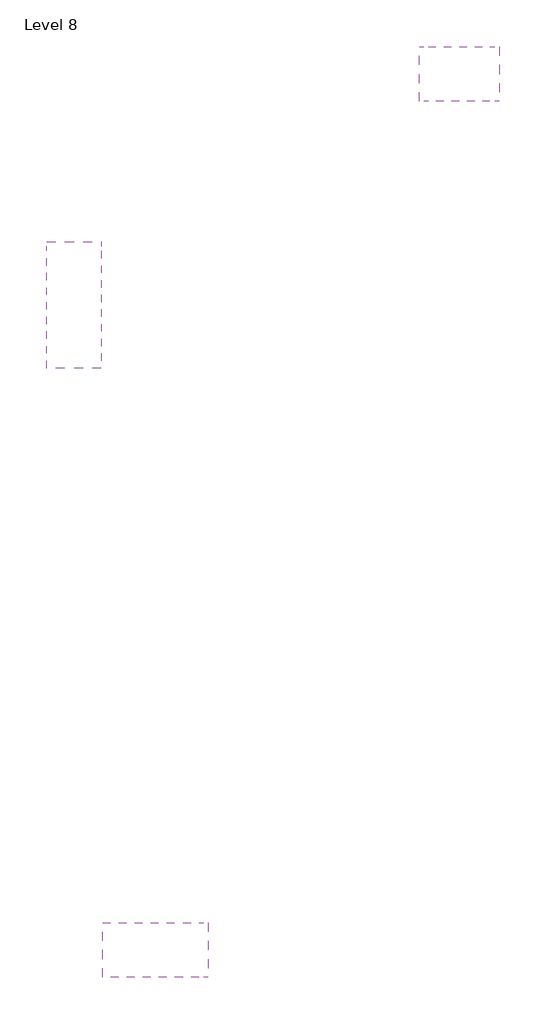
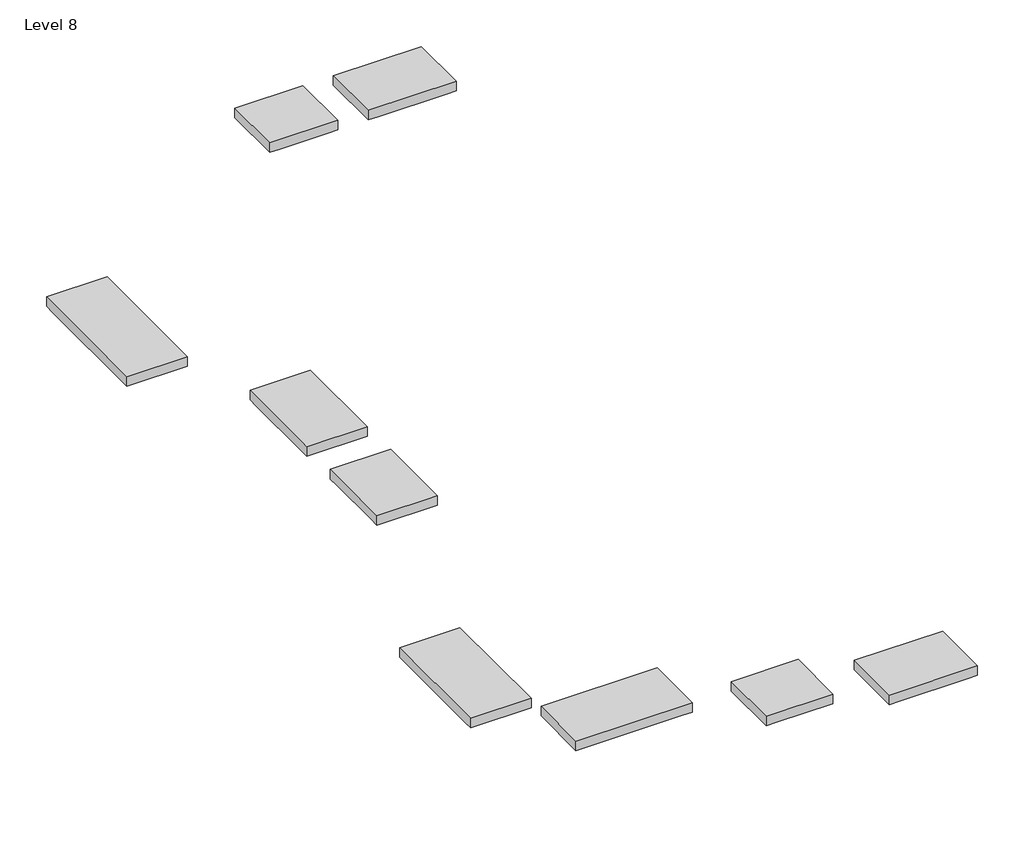
# One storey: 3 proxies.
"""IFC4 building model written with IfcOpenShell, lengths in millimetres."""

from ifc_helpers import new_model, si_unit, origin, place, context, project, spatial, transform, mapped, element, save
from components import generic_models_10_generic_models_10_998b1f2c, generic_models_11_generic_models_11_73ad1d2d, generic_models_12_generic_models_12_6034f315

model = new_model("IFC4")

# Units and contexts
model_context = context("Model", 3, world=origin())
ifc_project = project(units=[si_unit("LENGTHUNIT", "METRE", prefix="MILLI")], contexts=[model_context])

# Site, building, storey
site = spatial("IfcSite", under=ifc_project)
building = spatial("IfcBuilding", under=site)
storey = spatial("IfcBuildingStorey", under=building, Name="Level 8", Elevation=3962.4)

# Proxies
placement = place(None, origin())
generic_models_10_generic_models_10_shape = generic_models_10_generic_models_10_998b1f2c(model_context)
element("IfcBuildingElementProxy", 1, Name="Generic Models 10 : Generic Models 10", ObjectType="Generic Models 10 : Generic Models 10", at=placement, inside=storey, context=model_context, shape_type="MappedRepresentation", body=[
    mapped(generic_models_10_generic_models_10_shape, transform((0.0, 0.0, 0.0), x_axis=(1.0, 0.0, 0.0), y_axis=(0.0, 1.0, 0.0), z_axis=(0.0, 0.0, 1.0))),
])
generic_models_11_generic_models_11_shape = generic_models_11_generic_models_11_73ad1d2d(model_context)
element("IfcBuildingElementProxy", 2, Name="Generic Models 11 : Generic Models 11", ObjectType="Generic Models 11 : Generic Models 11", at=placement, inside=storey, context=model_context, shape_type="MappedRepresentation", body=[
    mapped(generic_models_11_generic_models_11_shape, transform((0.0, 0.0, 0.0), x_axis=(1.0, 0.0, 0.0), y_axis=(0.0, 1.0, 0.0), z_axis=(0.0, 0.0, 1.0))),
])
generic_models_12_generic_models_12_shape = generic_models_12_generic_models_12_6034f315(model_context)
element("IfcBuildingElementProxy", 3, Name="Generic Models 12 : Generic Models 12", ObjectType="Generic Models 12 : Generic Models 12", at=placement, inside=storey, context=model_context, shape_type="MappedRepresentation", body=[
    mapped(generic_models_12_generic_models_12_shape, transform((0.0, 0.0, 0.0), x_axis=(1.0, 0.0, 0.0), y_axis=(0.0, 1.0, 0.0), z_axis=(0.0, 0.0, 1.0))),
])

save(model, "model.ifc")

# Revit data of these elements
# Element 1 (IfcBuildingElementProxy, "Generic Models 10 : Generic Models 10")
#   Phase Created = New Construction
# Element 2 (IfcBuildingElementProxy, "Generic Models 11 : Generic Models 11")
#   Phase Created = New Construction
# Element 3 (IfcBuildingElementProxy, "Generic Models 12 : Generic Models 12")
#   Phase Created = New Construction
